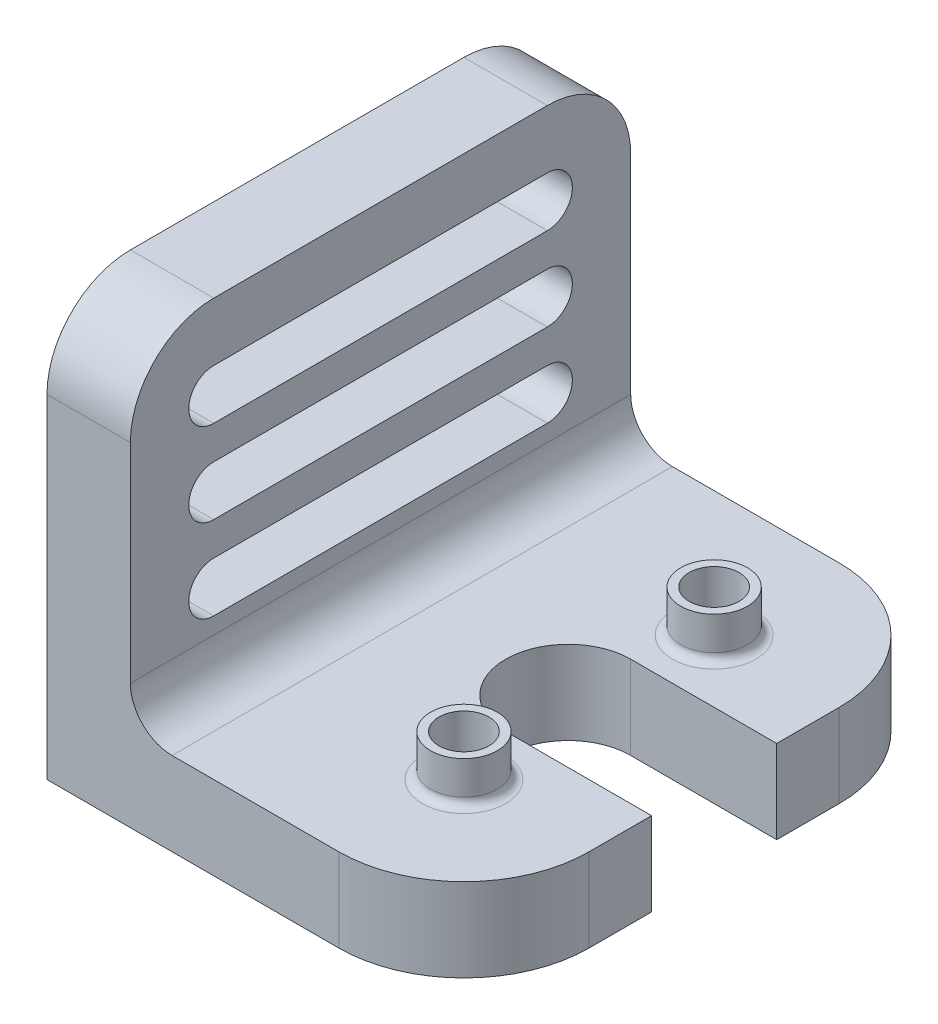
ISO-10303-21;
HEADER;
FILE_DESCRIPTION(('STEP AP214'),'2;1');
FILE_NAME('part.step','',(''),(''),'','','');
FILE_SCHEMA(('AUTOMOTIVE_DESIGN { 1 0 10303 214 1 1 1 1 }'));
ENDSEC;
DATA;
#1=APPLICATION_CONTEXT('core data for automotive mechanical design processes');
#2=APPLICATION_PROTOCOL_DEFINITION('international standard','automotive_design',2000,#1);
#3=PRODUCT_CONTEXT('',#1,'mechanical');
#4=PRODUCT('Part','Part','',(#3));
#5=PRODUCT_RELATED_PRODUCT_CATEGORY('part','',(#4));
#6=PRODUCT_DEFINITION_FORMATION('','',#4);
#7=PRODUCT_DEFINITION_CONTEXT('part definition',#1,'design');
#8=PRODUCT_DEFINITION('design','',#6,#7);
#9=PRODUCT_DEFINITION_SHAPE('','',#8);
#10=(LENGTH_UNIT() NAMED_UNIT(*) SI_UNIT(.MILLI.,.METRE.));
#11=(NAMED_UNIT(*) PLANE_ANGLE_UNIT() SI_UNIT($,.RADIAN.));
#12=(NAMED_UNIT(*) SI_UNIT($,.STERADIAN.) SOLID_ANGLE_UNIT());
#13=UNCERTAINTY_MEASURE_WITH_UNIT(LENGTH_MEASURE(1.E-05),#10,'distance_accuracy_value','');
#14=(GEOMETRIC_REPRESENTATION_CONTEXT(3) GLOBAL_UNCERTAINTY_ASSIGNED_CONTEXT((#13)) GLOBAL_UNIT_ASSIGNED_CONTEXT((#10,
#11,#12)) REPRESENTATION_CONTEXT('',''));
#15=CARTESIAN_POINT('',(0.,0.,0.));
#16=DIRECTION('',(0.,0.,1.));
#17=DIRECTION('',(1.,0.,0.));
#18=AXIS2_PLACEMENT_3D('',#15,#16,#17);
#19=CARTESIAN_POINT('',(100.,0.,60.));
#20=DIRECTION('',(-1.,0.,0.));
#21=DIRECTION('',(0.,0.,1.));
#22=AXIS2_PLACEMENT_3D('',#19,#20,#21);
#23=PLANE('',#22);
#24=DIRECTION('',(0.,0.,-1.));
#25=VECTOR('',#24,1.);
#26=CARTESIAN_POINT('',(100.,-80.,60.));
#27=LINE('',#26,#25);
#28=CARTESIAN_POINT('',(100.,-80.,-15.));
#29=VERTEX_POINT('',#28);
#30=CARTESIAN_POINT('',(100.,-80.,-30.));
#31=VERTEX_POINT('',#30);
#32=EDGE_CURVE('E357',#29,#31,#27,.T.);
#33=ORIENTED_EDGE('',*,*,#32,.F.);
#34=DIRECTION('',(0.,-1.,0.));
#35=VECTOR('',#34,1.);
#36=CARTESIAN_POINT('',(100.,0.,-15.));
#37=LINE('',#36,#35);
#38=CARTESIAN_POINT('',(100.,-100.,-15.));
#39=VERTEX_POINT('',#38);
#40=EDGE_CURVE('E427',#29,#39,#37,.T.);
#41=ORIENTED_EDGE('',*,*,#40,.T.);
#42=DIRECTION('',(0.,0.,-1.));
#43=VECTOR('',#42,1.);
#44=CARTESIAN_POINT('',(100.,-100.,60.));
#45=LINE('',#44,#43);
#46=CARTESIAN_POINT('',(100.,-100.,-30.));
#47=VERTEX_POINT('',#46);
#48=EDGE_CURVE('E375',#39,#47,#45,.T.);
#49=ORIENTED_EDGE('',*,*,#48,.T.);
#50=DIRECTION('',(0.,1.,0.));
#51=VECTOR('',#50,1.);
#52=CARTESIAN_POINT('',(100.,0.,-30.));
#53=LINE('',#52,#51);
#54=EDGE_CURVE('E394',#47,#31,#53,.T.);
#55=ORIENTED_EDGE('',*,*,#54,.T.);
#56=EDGE_LOOP('',(#33,#41,#49,#55));
#57=FACE_BOUND('',#56,.T.);
#58=ADVANCED_FACE('F41',(#57),#23,.F.);
#59=CARTESIAN_POINT('',(0.,-80.,60.));
#60=DIRECTION('',(0.,1.,0.));
#61=DIRECTION('',(0.,0.,1.));
#62=AXIS2_PLACEMENT_3D('',#59,#60,#61);
#63=PLANE('',#62);
#64=CARTESIAN_POINT('',(70.,-80.,-30.));
#65=DIRECTION('',(0.,1.,0.));
#66=DIRECTION('',(0.,0.,1.));
#67=AXIS2_PLACEMENT_3D('',#64,#65,#66);
#68=CIRCLE('',#67,10.);
#69=CARTESIAN_POINT('',(70.,-80.,-20.));
#70=VERTEX_POINT('',#69);
#71=EDGE_CURVE('E47',#70,#70,#68,.F.);
#72=ORIENTED_EDGE('',*,*,#71,.T.);
#73=EDGE_LOOP('',(#72));
#74=FACE_BOUND('',#73,.T.);
#75=CARTESIAN_POINT('',(70.,-80.,30.));
#76=DIRECTION('',(0.,1.,0.));
#77=DIRECTION('',(0.,0.,1.));
#78=AXIS2_PLACEMENT_3D('',#75,#76,#77);
#79=CIRCLE('',#78,10.);
#80=CARTESIAN_POINT('',(70.,-80.,40.));
#81=VERTEX_POINT('',#80);
#82=EDGE_CURVE('E437',#81,#81,#79,.F.);
#83=ORIENTED_EDGE('',*,*,#82,.T.);
#84=EDGE_LOOP('',(#83));
#85=FACE_BOUND('',#84,.T.);
#86=DIRECTION('',(-1.,0.,0.));
#87=VECTOR('',#86,1.);
#88=CARTESIAN_POINT('',(65.,-80.,-15.));
#89=LINE('',#88,#87);
#90=CARTESIAN_POINT('',(65.,-80.,-15.));
#91=VERTEX_POINT('',#90);
#92=EDGE_CURVE('E330',#29,#91,#89,.T.);
#93=ORIENTED_EDGE('',*,*,#92,.F.);
#94=ORIENTED_EDGE('',*,*,#32,.T.);
#95=CARTESIAN_POINT('',(70.,-80.,-30.));
#96=DIRECTION('',(0.,1.,0.));
#97=DIRECTION('',(0.,0.,1.));
#98=AXIS2_PLACEMENT_3D('',#95,#96,#97);
#99=CIRCLE('',#98,30.);
#100=CARTESIAN_POINT('',(70.,-80.,-60.));
#101=VERTEX_POINT('',#100);
#102=EDGE_CURVE('E399',#31,#101,#99,.T.);
#103=ORIENTED_EDGE('',*,*,#102,.T.);
#104=DIRECTION('',(1.,0.,0.));
#105=VECTOR('',#104,1.);
#106=CARTESIAN_POINT('',(0.,-80.,-60.));
#107=LINE('',#106,#105);
#108=CARTESIAN_POINT('',(30.0000000000001,-80.,-60.));
#109=VERTEX_POINT('',#108);
#110=EDGE_CURVE('E345',#109,#101,#107,.T.);
#111=ORIENTED_EDGE('',*,*,#110,.F.);
#112=DIRECTION('',(0.,0.,-1.));
#113=VECTOR('',#112,1.);
#114=CARTESIAN_POINT('',(30.0000000000001,-80.,60.));
#115=LINE('',#114,#113);
#116=CARTESIAN_POINT('',(30.0000000000001,-80.,60.));
#117=VERTEX_POINT('',#116);
#118=EDGE_CURVE('E389',#117,#109,#115,.T.);
#119=ORIENTED_EDGE('',*,*,#118,.F.);
#120=DIRECTION('',(1.,0.,0.));
#121=VECTOR('',#120,1.);
#122=CARTESIAN_POINT('',(0.,-80.,60.));
#123=LINE('',#122,#121);
#124=CARTESIAN_POINT('',(70.,-80.,60.));
#125=VERTEX_POINT('',#124);
#126=EDGE_CURVE('E344',#117,#125,#123,.T.);
#127=ORIENTED_EDGE('',*,*,#126,.T.);
#128=CARTESIAN_POINT('',(70.,-80.,30.));
#129=DIRECTION('',(0.,1.,0.));
#130=DIRECTION('',(0.,0.,1.));
#131=AXIS2_PLACEMENT_3D('',#128,#129,#130);
#132=CIRCLE('',#131,30.);
#133=CARTESIAN_POINT('',(100.,-80.,30.));
#134=VERTEX_POINT('',#133);
#135=EDGE_CURVE('E391',#125,#134,#132,.T.);
#136=ORIENTED_EDGE('',*,*,#135,.T.);
#137=CARTESIAN_POINT('',(100.,-80.,15.));
#138=VERTEX_POINT('',#137);
#139=EDGE_CURVE('E367',#134,#138,#27,.T.);
#140=ORIENTED_EDGE('',*,*,#139,.T.);
#141=DIRECTION('',(1.,0.,0.));
#142=VECTOR('',#141,1.);
#143=CARTESIAN_POINT('',(100.,-80.,15.));
#144=LINE('',#143,#142);
#145=CARTESIAN_POINT('',(65.,-80.,15.));
#146=VERTEX_POINT('',#145);
#147=EDGE_CURVE('E329',#146,#138,#144,.T.);
#148=ORIENTED_EDGE('',*,*,#147,.F.);
#149=CARTESIAN_POINT('',(65.,-80.,0.));
#150=DIRECTION('',(0.,1.,0.));
#151=DIRECTION('',(0.,0.,-1.));
#152=AXIS2_PLACEMENT_3D('',#149,#150,#151);
#153=CIRCLE('',#152,15.);
#154=EDGE_CURVE('E256',#91,#146,#153,.T.);
#155=ORIENTED_EDGE('',*,*,#154,.F.);
#156=EDGE_LOOP('',(#93,#94,#103,#111,#119,#127,#136,#140,#148,#155));
#157=FACE_BOUND('',#156,.T.);
#158=ADVANCED_FACE('F443',(#74,#85,#157),#63,.T.);
#159=CARTESIAN_POINT('',(30.,-70.,60.));
#160=DIRECTION('',(0.,0.,-1.));
#161=DIRECTION('',(-1.,0.,0.));
#162=AXIS2_PLACEMENT_3D('',#159,#160,#161);
#163=CYLINDRICAL_SURFACE('',#162,10.);
#164=CARTESIAN_POINT('',(30.,-70.,-60.));
#165=DIRECTION('',(0.,0.,1.));
#166=DIRECTION('',(1.,0.,0.));
#167=AXIS2_PLACEMENT_3D('',#164,#165,#166);
#168=CIRCLE('',#167,10.);
#169=CARTESIAN_POINT('',(20.,-70.,-60.));
#170=VERTEX_POINT('',#169);
#171=EDGE_CURVE('E359',#109,#170,#168,.F.);
#172=ORIENTED_EDGE('',*,*,#171,.T.);
#173=DIRECTION('',(0.,0.,-1.));
#174=VECTOR('',#173,1.);
#175=CARTESIAN_POINT('',(20.,-70.,60.));
#176=LINE('',#175,#174);
#177=CARTESIAN_POINT('',(20.,-70.,60.));
#178=VERTEX_POINT('',#177);
#179=EDGE_CURVE('E383',#178,#170,#176,.T.);
#180=ORIENTED_EDGE('',*,*,#179,.F.);
#181=CARTESIAN_POINT('',(30.,-70.,60.));
#182=DIRECTION('',(0.,0.,1.));
#183=DIRECTION('',(1.,0.,0.));
#184=AXIS2_PLACEMENT_3D('',#181,#182,#183);
#185=CIRCLE('',#184,10.);
#186=EDGE_CURVE('E348',#117,#178,#185,.F.);
#187=ORIENTED_EDGE('',*,*,#186,.F.);
#188=ORIENTED_EDGE('',*,*,#118,.T.);
#189=EDGE_LOOP('',(#172,#180,#187,#188));
#190=FACE_BOUND('',#189,.T.);
#191=ADVANCED_FACE('F501',(#190),#163,.F.);
#192=CARTESIAN_POINT('',(20.,0.,60.));
#193=DIRECTION('',(1.,0.,0.));
#194=DIRECTION('',(0.,1.,0.));
#195=AXIS2_PLACEMENT_3D('',#192,#193,#194);
#196=PLANE('',#195);
#197=CARTESIAN_POINT('',(20.,-20.,40.));
#198=DIRECTION('',(1.,0.,0.));
#199=DIRECTION('',(0.,1.,0.));
#200=AXIS2_PLACEMENT_3D('',#197,#198,#199);
#201=CIRCLE('',#200,6.);
#202=CARTESIAN_POINT('',(20.,-14.,40.));
#203=VERTEX_POINT('',#202);
#204=CARTESIAN_POINT('',(20.,-26.,40.));
#205=VERTEX_POINT('',#204);
#206=EDGE_CURVE('E57',#203,#205,#201,.T.);
#207=ORIENTED_EDGE('',*,*,#206,.F.);
#208=DIRECTION('',(0.,0.,1.));
#209=VECTOR('',#208,1.);
#210=CARTESIAN_POINT('',(20.,-14.,40.));
#211=LINE('',#210,#209);
#212=CARTESIAN_POINT('',(20.,-14.,-40.));
#213=VERTEX_POINT('',#212);
#214=EDGE_CURVE('E241',#213,#203,#211,.T.);
#215=ORIENTED_EDGE('',*,*,#214,.F.);
#216=CARTESIAN_POINT('',(20.,-20.,-40.));
#217=DIRECTION('',(1.,0.,0.));
#218=DIRECTION('',(0.,1.,0.));
#219=AXIS2_PLACEMENT_3D('',#216,#217,#218);
#220=CIRCLE('',#219,6.);
#221=CARTESIAN_POINT('',(20.,-26.,-40.));
#222=VERTEX_POINT('',#221);
#223=EDGE_CURVE('E242',#222,#213,#220,.T.);
#224=ORIENTED_EDGE('',*,*,#223,.F.);
#225=DIRECTION('',(0.,0.,-1.));
#226=VECTOR('',#225,1.);
#227=CARTESIAN_POINT('',(20.,-26.,40.));
#228=LINE('',#227,#226);
#229=EDGE_CURVE('E254',#205,#222,#228,.T.);
#230=ORIENTED_EDGE('',*,*,#229,.F.);
#231=EDGE_LOOP('',(#207,#215,#224,#230));
#232=FACE_BOUND('',#231,.T.);
#233=CARTESIAN_POINT('',(20.,-40.,39.9999999999998));
#234=DIRECTION('',(1.,0.,0.));
#235=DIRECTION('',(0.,1.,0.));
#236=AXIS2_PLACEMENT_3D('',#233,#234,#235);
#237=CIRCLE('',#236,6.);
#238=CARTESIAN_POINT('',(20.,-34.,39.9999999999998));
#239=VERTEX_POINT('',#238);
#240=CARTESIAN_POINT('',(20.,-46.,39.9999999999998));
#241=VERTEX_POINT('',#240);
#242=EDGE_CURVE('E61',#239,#241,#237,.T.);
#243=ORIENTED_EDGE('',*,*,#242,.F.);
#244=DIRECTION('',(0.,0.,1.));
#245=VECTOR('',#244,1.);
#246=CARTESIAN_POINT('',(20.,-34.,39.9999999999998));
#247=LINE('',#246,#245);
#248=CARTESIAN_POINT('',(20.,-34.,-40.0000000000002));
#249=VERTEX_POINT('',#248);
#250=EDGE_CURVE('E271',#249,#239,#247,.T.);
#251=ORIENTED_EDGE('',*,*,#250,.F.);
#252=CARTESIAN_POINT('',(20.,-40.,-40.0000000000002));
#253=DIRECTION('',(1.,0.,0.));
#254=DIRECTION('',(0.,1.,0.));
#255=AXIS2_PLACEMENT_3D('',#252,#253,#254);
#256=CIRCLE('',#255,6.);
#257=CARTESIAN_POINT('',(20.,-46.,-40.0000000000002));
#258=VERTEX_POINT('',#257);
#259=EDGE_CURVE('E277',#258,#249,#256,.T.);
#260=ORIENTED_EDGE('',*,*,#259,.F.);
#261=DIRECTION('',(0.,0.,-1.));
#262=VECTOR('',#261,1.);
#263=CARTESIAN_POINT('',(20.,-46.,39.9999999999998));
#264=LINE('',#263,#262);
#265=EDGE_CURVE('E278',#241,#258,#264,.T.);
#266=ORIENTED_EDGE('',*,*,#265,.F.);
#267=EDGE_LOOP('',(#243,#251,#260,#266));
#268=FACE_BOUND('',#267,.T.);
#269=CARTESIAN_POINT('',(20.,-60.,39.9999999999996));
#270=DIRECTION('',(1.,0.,0.));
#271=DIRECTION('',(0.,1.,0.));
#272=AXIS2_PLACEMENT_3D('',#269,#270,#271);
#273=CIRCLE('',#272,6.);
#274=CARTESIAN_POINT('',(20.,-54.,39.9999999999996));
#275=VERTEX_POINT('',#274);
#276=CARTESIAN_POINT('',(20.,-66.,39.9999999999996));
#277=VERTEX_POINT('',#276);
#278=EDGE_CURVE('E275',#275,#277,#273,.T.);
#279=ORIENTED_EDGE('',*,*,#278,.F.);
#280=DIRECTION('',(0.,0.,1.));
#281=VECTOR('',#280,1.);
#282=CARTESIAN_POINT('',(20.,-54.,39.9999999999996));
#283=LINE('',#282,#281);
#284=CARTESIAN_POINT('',(20.,-54.,-40.0000000000004));
#285=VERTEX_POINT('',#284);
#286=EDGE_CURVE('E302',#285,#275,#283,.T.);
#287=ORIENTED_EDGE('',*,*,#286,.F.);
#288=CARTESIAN_POINT('',(20.,-60.,-40.0000000000004));
#289=DIRECTION('',(1.,0.,0.));
#290=DIRECTION('',(0.,1.,0.));
#291=AXIS2_PLACEMENT_3D('',#288,#289,#290);
#292=CIRCLE('',#291,6.);
#293=CARTESIAN_POINT('',(20.,-66.,-40.0000000000004));
#294=VERTEX_POINT('',#293);
#295=EDGE_CURVE('E310',#294,#285,#292,.T.);
#296=ORIENTED_EDGE('',*,*,#295,.F.);
#297=DIRECTION('',(0.,0.,-1.));
#298=VECTOR('',#297,1.);
#299=CARTESIAN_POINT('',(20.,-66.,39.9999999999996));
#300=LINE('',#299,#298);
#301=EDGE_CURVE('E311',#277,#294,#300,.T.);
#302=ORIENTED_EDGE('',*,*,#301,.F.);
#303=EDGE_LOOP('',(#279,#287,#296,#302));
#304=FACE_BOUND('',#303,.T.);
#305=DIRECTION('',(0.,-1.,0.));
#306=VECTOR('',#305,1.);
#307=CARTESIAN_POINT('',(20.,0.,-60.));
#308=LINE('',#307,#306);
#309=CARTESIAN_POINT('',(20.,-20.,-60.));
#310=VERTEX_POINT('',#309);
#311=EDGE_CURVE('E361',#310,#170,#308,.T.);
#312=ORIENTED_EDGE('',*,*,#311,.F.);
#313=CARTESIAN_POINT('',(20.,-20.,-40.));
#314=DIRECTION('',(1.,0.,0.));
#315=DIRECTION('',(0.,1.,0.));
#316=AXIS2_PLACEMENT_3D('',#313,#314,#315);
#317=CIRCLE('',#316,20.);
#318=CARTESIAN_POINT('',(20.,0.,-40.));
#319=VERTEX_POINT('',#318);
#320=EDGE_CURVE('E415',#310,#319,#317,.T.);
#321=ORIENTED_EDGE('',*,*,#320,.T.);
#322=DIRECTION('',(0.,0.,-1.));
#323=VECTOR('',#322,1.);
#324=CARTESIAN_POINT('',(20.,0.,60.));
#325=LINE('',#324,#323);
#326=CARTESIAN_POINT('',(20.,0.,40.));
#327=VERTEX_POINT('',#326);
#328=EDGE_CURVE('E385',#327,#319,#325,.T.);
#329=ORIENTED_EDGE('',*,*,#328,.F.);
#330=CARTESIAN_POINT('',(20.,-20.,40.));
#331=DIRECTION('',(1.,0.,0.));
#332=DIRECTION('',(0.,1.,0.));
#333=AXIS2_PLACEMENT_3D('',#330,#331,#332);
#334=CIRCLE('',#333,20.);
#335=CARTESIAN_POINT('',(20.,-20.,60.));
#336=VERTEX_POINT('',#335);
#337=EDGE_CURVE('E414',#327,#336,#334,.T.);
#338=ORIENTED_EDGE('',*,*,#337,.T.);
#339=DIRECTION('',(0.,-1.,0.));
#340=VECTOR('',#339,1.);
#341=CARTESIAN_POINT('',(20.,0.,60.));
#342=LINE('',#341,#340);
#343=EDGE_CURVE('E346',#336,#178,#342,.T.);
#344=ORIENTED_EDGE('',*,*,#343,.T.);
#345=ORIENTED_EDGE('',*,*,#179,.T.);
#346=EDGE_LOOP('',(#312,#321,#329,#338,#344,#345));
#347=FACE_BOUND('',#346,.T.);
#348=ADVANCED_FACE('F573',(#232,#268,#304,#347),#196,.T.);
#349=CARTESIAN_POINT('',(0.,0.,60.));
#350=DIRECTION('',(0.,1.,0.));
#351=DIRECTION('',(0.,0.,1.));
#352=AXIS2_PLACEMENT_3D('',#349,#350,#351);
#353=PLANE('',#352);
#354=ORIENTED_EDGE('',*,*,#328,.T.);
#355=DIRECTION('',(1.,0.,0.));
#356=VECTOR('',#355,1.);
#357=CARTESIAN_POINT('',(0.,0.,-40.));
#358=LINE('',#357,#356);
#359=CARTESIAN_POINT('',(0.,0.,-40.));
#360=VERTEX_POINT('',#359);
#361=EDGE_CURVE('E416',#319,#360,#358,.F.);
#362=ORIENTED_EDGE('',*,*,#361,.T.);
#363=DIRECTION('',(0.,0.,-1.));
#364=VECTOR('',#363,1.);
#365=CARTESIAN_POINT('',(0.,0.,60.));
#366=LINE('',#365,#364);
#367=CARTESIAN_POINT('',(0.,0.,40.));
#368=VERTEX_POINT('',#367);
#369=EDGE_CURVE('E378',#368,#360,#366,.T.);
#370=ORIENTED_EDGE('',*,*,#369,.F.);
#371=DIRECTION('',(1.,0.,0.));
#372=VECTOR('',#371,1.);
#373=CARTESIAN_POINT('',(0.,0.,40.));
#374=LINE('',#373,#372);
#375=EDGE_CURVE('E417',#368,#327,#374,.T.);
#376=ORIENTED_EDGE('',*,*,#375,.T.);
#377=EDGE_LOOP('',(#354,#362,#370,#376));
#378=FACE_BOUND('',#377,.T.);
#379=ADVANCED_FACE('F550',(#378),#353,.T.);
#380=CARTESIAN_POINT('',(0.,0.,60.));
#381=DIRECTION('',(1.,0.,0.));
#382=DIRECTION('',(0.,0.,-1.));
#383=AXIS2_PLACEMENT_3D('',#380,#381,#382);
#384=PLANE('',#383);
#385=DIRECTION('',(0.,0.,1.));
#386=VECTOR('',#385,1.);
#387=CARTESIAN_POINT('',(0.,-14.,40.));
#388=LINE('',#387,#386);
#389=CARTESIAN_POINT('',(0.,-14.,-40.));
#390=VERTEX_POINT('',#389);
#391=CARTESIAN_POINT('',(0.,-14.,40.));
#392=VERTEX_POINT('',#391);
#393=EDGE_CURVE('E226',#390,#392,#388,.T.);
#394=ORIENTED_EDGE('',*,*,#393,.T.);
#395=CARTESIAN_POINT('',(0.,-20.,40.));
#396=DIRECTION('',(1.,0.,0.));
#397=DIRECTION('',(0.,1.,0.));
#398=AXIS2_PLACEMENT_3D('',#395,#396,#397);
#399=CIRCLE('',#398,6.);
#400=CARTESIAN_POINT('',(0.,-26.,40.));
#401=VERTEX_POINT('',#400);
#402=EDGE_CURVE('E224',#392,#401,#399,.T.);
#403=ORIENTED_EDGE('',*,*,#402,.T.);
#404=DIRECTION('',(0.,0.,-1.));
#405=VECTOR('',#404,1.);
#406=CARTESIAN_POINT('',(0.,-26.,40.));
#407=LINE('',#406,#405);
#408=CARTESIAN_POINT('',(0.,-26.,-40.));
#409=VERTEX_POINT('',#408);
#410=EDGE_CURVE('E235',#401,#409,#407,.T.);
#411=ORIENTED_EDGE('',*,*,#410,.T.);
#412=CARTESIAN_POINT('',(0.,-20.,-40.));
#413=DIRECTION('',(1.,0.,0.));
#414=DIRECTION('',(0.,1.,0.));
#415=AXIS2_PLACEMENT_3D('',#412,#413,#414);
#416=CIRCLE('',#415,6.);
#417=EDGE_CURVE('E236',#409,#390,#416,.T.);
#418=ORIENTED_EDGE('',*,*,#417,.T.);
#419=EDGE_LOOP('',(#394,#403,#411,#418));
#420=FACE_BOUND('',#419,.T.);
#421=DIRECTION('',(0.,0.,1.));
#422=VECTOR('',#421,1.);
#423=CARTESIAN_POINT('',(0.,-34.,39.9999999999998));
#424=LINE('',#423,#422);
#425=CARTESIAN_POINT('',(0.,-34.,-40.0000000000002));
#426=VERTEX_POINT('',#425);
#427=CARTESIAN_POINT('',(0.,-34.,39.9999999999998));
#428=VERTEX_POINT('',#427);
#429=EDGE_CURVE('E261',#426,#428,#424,.T.);
#430=ORIENTED_EDGE('',*,*,#429,.T.);
#431=CARTESIAN_POINT('',(0.,-40.,39.9999999999998));
#432=DIRECTION('',(1.,0.,0.));
#433=DIRECTION('',(0.,1.,0.));
#434=AXIS2_PLACEMENT_3D('',#431,#432,#433);
#435=CIRCLE('',#434,6.);
#436=CARTESIAN_POINT('',(0.,-46.,39.9999999999998));
#437=VERTEX_POINT('',#436);
#438=EDGE_CURVE('E280',#428,#437,#435,.T.);
#439=ORIENTED_EDGE('',*,*,#438,.T.);
#440=DIRECTION('',(0.,0.,-1.));
#441=VECTOR('',#440,1.);
#442=CARTESIAN_POINT('',(0.,-46.,39.9999999999998));
#443=LINE('',#442,#441);
#444=CARTESIAN_POINT('',(0.,-46.,-40.0000000000002));
#445=VERTEX_POINT('',#444);
#446=EDGE_CURVE('E286',#437,#445,#443,.T.);
#447=ORIENTED_EDGE('',*,*,#446,.T.);
#448=CARTESIAN_POINT('',(0.,-40.,-40.0000000000002));
#449=DIRECTION('',(1.,0.,0.));
#450=DIRECTION('',(0.,1.,0.));
#451=AXIS2_PLACEMENT_3D('',#448,#449,#450);
#452=CIRCLE('',#451,6.);
#453=EDGE_CURVE('E287',#445,#426,#452,.T.);
#454=ORIENTED_EDGE('',*,*,#453,.T.);
#455=EDGE_LOOP('',(#430,#439,#447,#454));
#456=FACE_BOUND('',#455,.T.);
#457=DIRECTION('',(0.,0.,1.));
#458=VECTOR('',#457,1.);
#459=CARTESIAN_POINT('',(0.,-54.,39.9999999999996));
#460=LINE('',#459,#458);
#461=CARTESIAN_POINT('',(0.,-54.,-40.0000000000004));
#462=VERTEX_POINT('',#461);
#463=CARTESIAN_POINT('',(0.,-54.,39.9999999999996));
#464=VERTEX_POINT('',#463);
#465=EDGE_CURVE('E300',#462,#464,#460,.T.);
#466=ORIENTED_EDGE('',*,*,#465,.T.);
#467=CARTESIAN_POINT('',(0.,-60.,39.9999999999996));
#468=DIRECTION('',(1.,0.,0.));
#469=DIRECTION('',(0.,1.,0.));
#470=AXIS2_PLACEMENT_3D('',#467,#468,#469);
#471=CIRCLE('',#470,6.);
#472=CARTESIAN_POINT('',(0.,-66.,39.9999999999996));
#473=VERTEX_POINT('',#472);
#474=EDGE_CURVE('E308',#464,#473,#471,.T.);
#475=ORIENTED_EDGE('',*,*,#474,.T.);
#476=DIRECTION('',(0.,0.,-1.));
#477=VECTOR('',#476,1.);
#478=CARTESIAN_POINT('',(0.,-66.,39.9999999999996));
#479=LINE('',#478,#477);
#480=CARTESIAN_POINT('',(0.,-66.,-40.0000000000004));
#481=VERTEX_POINT('',#480);
#482=EDGE_CURVE('E318',#473,#481,#479,.T.);
#483=ORIENTED_EDGE('',*,*,#482,.T.);
#484=CARTESIAN_POINT('',(0.,-60.,-40.0000000000004));
#485=DIRECTION('',(1.,0.,0.));
#486=DIRECTION('',(0.,1.,0.));
#487=AXIS2_PLACEMENT_3D('',#484,#485,#486);
#488=CIRCLE('',#487,6.);
#489=EDGE_CURVE('E320',#481,#462,#488,.T.);
#490=ORIENTED_EDGE('',*,*,#489,.T.);
#491=EDGE_LOOP('',(#466,#475,#483,#490));
#492=FACE_BOUND('',#491,.T.);
#493=ORIENTED_EDGE('',*,*,#369,.T.);
#494=CARTESIAN_POINT('',(0.,-20.,-40.));
#495=DIRECTION('',(1.,0.,0.));
#496=DIRECTION('',(0.,0.,-1.));
#497=AXIS2_PLACEMENT_3D('',#494,#495,#496);
#498=CIRCLE('',#497,20.);
#499=CARTESIAN_POINT('',(0.,-20.,-60.));
#500=VERTEX_POINT('',#499);
#501=EDGE_CURVE('E421',#360,#500,#498,.F.);
#502=ORIENTED_EDGE('',*,*,#501,.T.);
#503=DIRECTION('',(0.,-1.,0.));
#504=VECTOR('',#503,1.);
#505=CARTESIAN_POINT('',(0.,0.,-60.));
#506=LINE('',#505,#504);
#507=CARTESIAN_POINT('',(0.,-100.,-60.));
#508=VERTEX_POINT('',#507);
#509=EDGE_CURVE('E362',#500,#508,#506,.T.);
#510=ORIENTED_EDGE('',*,*,#509,.T.);
#511=DIRECTION('',(0.,0.,-1.));
#512=VECTOR('',#511,1.);
#513=CARTESIAN_POINT('',(0.,-100.,60.));
#514=LINE('',#513,#512);
#515=CARTESIAN_POINT('',(0.,-100.,60.));
#516=VERTEX_POINT('',#515);
#517=EDGE_CURVE('E376',#516,#508,#514,.T.);
#518=ORIENTED_EDGE('',*,*,#517,.F.);
#519=DIRECTION('',(0.,-1.,0.));
#520=VECTOR('',#519,1.);
#521=CARTESIAN_POINT('',(0.,0.,60.));
#522=LINE('',#521,#520);
#523=CARTESIAN_POINT('',(0.,-20.,60.));
#524=VERTEX_POINT('',#523);
#525=EDGE_CURVE('E354',#524,#516,#522,.T.);
#526=ORIENTED_EDGE('',*,*,#525,.F.);
#527=CARTESIAN_POINT('',(0.,-20.,40.));
#528=DIRECTION('',(1.,0.,0.));
#529=DIRECTION('',(0.,0.,-1.));
#530=AXIS2_PLACEMENT_3D('',#527,#528,#529);
#531=CIRCLE('',#530,20.);
#532=EDGE_CURVE('E423',#524,#368,#531,.F.);
#533=ORIENTED_EDGE('',*,*,#532,.T.);
#534=EDGE_LOOP('',(#493,#502,#510,#518,#526,#533));
#535=FACE_BOUND('',#534,.T.);
#536=ADVANCED_FACE('F238',(#420,#456,#492,#535),#384,.F.);
#537=CARTESIAN_POINT('',(0.,-100.,60.));
#538=DIRECTION('',(0.,1.,0.));
#539=DIRECTION('',(0.,0.,1.));
#540=AXIS2_PLACEMENT_3D('',#537,#538,#539);
#541=PLANE('',#540);
#542=ORIENTED_EDGE('',*,*,#48,.F.);
#543=DIRECTION('',(-1.,0.,0.));
#544=VECTOR('',#543,1.);
#545=CARTESIAN_POINT('',(0.,-100.,-15.));
#546=LINE('',#545,#544);
#547=CARTESIAN_POINT('',(65.,-100.,-15.));
#548=VERTEX_POINT('',#547);
#549=EDGE_CURVE('E339',#39,#548,#546,.T.);
#550=ORIENTED_EDGE('',*,*,#549,.T.);
#551=CARTESIAN_POINT('',(65.,-100.,0.));
#552=DIRECTION('',(0.,1.,0.));
#553=DIRECTION('',(0.,0.,1.));
#554=AXIS2_PLACEMENT_3D('',#551,#552,#553);
#555=CIRCLE('',#554,15.);
#556=CARTESIAN_POINT('',(65.,-100.,15.));
#557=VERTEX_POINT('',#556);
#558=EDGE_CURVE('E433',#548,#557,#555,.T.);
#559=ORIENTED_EDGE('',*,*,#558,.T.);
#560=DIRECTION('',(1.,0.,0.));
#561=VECTOR('',#560,1.);
#562=CARTESIAN_POINT('',(0.,-100.,15.));
#563=LINE('',#562,#561);
#564=CARTESIAN_POINT('',(100.,-100.,15.));
#565=VERTEX_POINT('',#564);
#566=EDGE_CURVE('E333',#557,#565,#563,.T.);
#567=ORIENTED_EDGE('',*,*,#566,.T.);
#568=CARTESIAN_POINT('',(100.,-100.,30.));
#569=VERTEX_POINT('',#568);
#570=EDGE_CURVE('E373',#569,#565,#45,.T.);
#571=ORIENTED_EDGE('',*,*,#570,.F.);
#572=CARTESIAN_POINT('',(70.,-100.,30.));
#573=DIRECTION('',(0.,1.,0.));
#574=DIRECTION('',(0.,0.,1.));
#575=AXIS2_PLACEMENT_3D('',#572,#573,#574);
#576=CIRCLE('',#575,30.);
#577=CARTESIAN_POINT('',(70.,-100.,60.));
#578=VERTEX_POINT('',#577);
#579=EDGE_CURVE('E402',#569,#578,#576,.F.);
#580=ORIENTED_EDGE('',*,*,#579,.T.);
#581=DIRECTION('',(1.,0.,0.));
#582=VECTOR('',#581,1.);
#583=CARTESIAN_POINT('',(0.,-100.,60.));
#584=LINE('',#583,#582);
#585=EDGE_CURVE('E351',#516,#578,#584,.T.);
#586=ORIENTED_EDGE('',*,*,#585,.F.);
#587=ORIENTED_EDGE('',*,*,#517,.T.);
#588=DIRECTION('',(1.,0.,0.));
#589=VECTOR('',#588,1.);
#590=CARTESIAN_POINT('',(0.,-100.,-60.));
#591=LINE('',#590,#589);
#592=CARTESIAN_POINT('',(70.,-100.,-60.));
#593=VERTEX_POINT('',#592);
#594=EDGE_CURVE('E349',#508,#593,#591,.T.);
#595=ORIENTED_EDGE('',*,*,#594,.T.);
#596=CARTESIAN_POINT('',(70.,-100.,-30.));
#597=DIRECTION('',(0.,1.,0.));
#598=DIRECTION('',(0.,0.,1.));
#599=AXIS2_PLACEMENT_3D('',#596,#597,#598);
#600=CIRCLE('',#599,30.);
#601=EDGE_CURVE('E401',#593,#47,#600,.F.);
#602=ORIENTED_EDGE('',*,*,#601,.T.);
#603=EDGE_LOOP('',(#542,#550,#559,#567,#571,#580,#586,#587,#595,#602));
#604=FACE_BOUND('',#603,.T.);
#605=ADVANCED_FACE('F507',(#604),#541,.F.);
#606=ORIENTED_EDGE('',*,*,#570,.T.);
#607=DIRECTION('',(0.,1.,0.));
#608=VECTOR('',#607,1.);
#609=CARTESIAN_POINT('',(100.,0.,15.));
#610=LINE('',#609,#608);
#611=EDGE_CURVE('E430',#565,#138,#610,.T.);
#612=ORIENTED_EDGE('',*,*,#611,.T.);
#613=ORIENTED_EDGE('',*,*,#139,.F.);
#614=DIRECTION('',(0.,1.,0.));
#615=VECTOR('',#614,1.);
#616=CARTESIAN_POINT('',(100.,-100.,30.));
#617=LINE('',#616,#615);
#618=EDGE_CURVE('E388',#134,#569,#617,.F.);
#619=ORIENTED_EDGE('',*,*,#618,.T.);
#620=EDGE_LOOP('',(#606,#612,#613,#619));
#621=FACE_BOUND('',#620,.T.);
#622=ADVANCED_FACE('F492',(#621),#23,.F.);
#623=CARTESIAN_POINT('',(0.,0.,60.));
#624=DIRECTION('',(0.,0.,1.));
#625=DIRECTION('',(1.,0.,0.));
#626=AXIS2_PLACEMENT_3D('',#623,#624,#625);
#627=PLANE('',#626);
#628=ORIENTED_EDGE('',*,*,#343,.F.);
#629=DIRECTION('',(1.,0.,0.));
#630=VECTOR('',#629,1.);
#631=CARTESIAN_POINT('',(0.,-20.,60.));
#632=LINE('',#631,#630);
#633=EDGE_CURVE('E424',#336,#524,#632,.F.);
#634=ORIENTED_EDGE('',*,*,#633,.T.);
#635=ORIENTED_EDGE('',*,*,#525,.T.);
#636=ORIENTED_EDGE('',*,*,#585,.T.);
#637=DIRECTION('',(0.,1.,0.));
#638=VECTOR('',#637,1.);
#639=CARTESIAN_POINT('',(70.,-80.,60.));
#640=LINE('',#639,#638);
#641=EDGE_CURVE('E407',#578,#125,#640,.T.);
#642=ORIENTED_EDGE('',*,*,#641,.T.);
#643=ORIENTED_EDGE('',*,*,#126,.F.);
#644=ORIENTED_EDGE('',*,*,#186,.T.);
#645=EDGE_LOOP('',(#628,#634,#635,#636,#642,#643,#644));
#646=FACE_BOUND('',#645,.T.);
#647=ADVANCED_FACE('F510',(#646),#627,.T.);
#648=CARTESIAN_POINT('',(0.,0.,-60.));
#649=DIRECTION('',(0.,0.,1.));
#650=DIRECTION('',(1.,0.,0.));
#651=AXIS2_PLACEMENT_3D('',#648,#649,#650);
#652=PLANE('',#651);
#653=ORIENTED_EDGE('',*,*,#509,.F.);
#654=DIRECTION('',(1.,0.,0.));
#655=VECTOR('',#654,1.);
#656=CARTESIAN_POINT('',(20.,-20.,-60.));
#657=LINE('',#656,#655);
#658=EDGE_CURVE('E406',#500,#310,#657,.T.);
#659=ORIENTED_EDGE('',*,*,#658,.T.);
#660=ORIENTED_EDGE('',*,*,#311,.T.);
#661=ORIENTED_EDGE('',*,*,#171,.F.);
#662=ORIENTED_EDGE('',*,*,#110,.T.);
#663=DIRECTION('',(0.,1.,0.));
#664=VECTOR('',#663,1.);
#665=CARTESIAN_POINT('',(70.,0.,-60.));
#666=LINE('',#665,#664);
#667=EDGE_CURVE('E396',#101,#593,#666,.F.);
#668=ORIENTED_EDGE('',*,*,#667,.T.);
#669=ORIENTED_EDGE('',*,*,#594,.F.);
#670=EDGE_LOOP('',(#653,#659,#660,#661,#662,#668,#669));
#671=FACE_BOUND('',#670,.T.);
#672=ADVANCED_FACE('F511',(#671),#652,.F.);
#673=CARTESIAN_POINT('',(70.,0.,-30.));
#674=DIRECTION('',(0.,1.,0.));
#675=DIRECTION('',(0.,0.,1.));
#676=AXIS2_PLACEMENT_3D('',#673,#674,#675);
#677=CYLINDRICAL_SURFACE('',#676,30.);
#678=ORIENTED_EDGE('',*,*,#601,.F.);
#679=ORIENTED_EDGE('',*,*,#667,.F.);
#680=ORIENTED_EDGE('',*,*,#102,.F.);
#681=ORIENTED_EDGE('',*,*,#54,.F.);
#682=EDGE_LOOP('',(#678,#679,#680,#681));
#683=FACE_BOUND('',#682,.T.);
#684=ADVANCED_FACE('F565',(#683),#677,.T.);
#685=CARTESIAN_POINT('',(70.,0.,30.));
#686=DIRECTION('',(0.,-1.,0.));
#687=DIRECTION('',(0.,0.,-1.));
#688=AXIS2_PLACEMENT_3D('',#685,#686,#687);
#689=CYLINDRICAL_SURFACE('',#688,30.);
#690=ORIENTED_EDGE('',*,*,#579,.F.);
#691=ORIENTED_EDGE('',*,*,#618,.F.);
#692=ORIENTED_EDGE('',*,*,#135,.F.);
#693=ORIENTED_EDGE('',*,*,#641,.F.);
#694=EDGE_LOOP('',(#690,#691,#692,#693));
#695=FACE_BOUND('',#694,.T.);
#696=ADVANCED_FACE('F527',(#695),#689,.T.);
#697=CARTESIAN_POINT('',(0.,-20.,-40.));
#698=DIRECTION('',(-1.,0.,0.));
#699=DIRECTION('',(0.,0.,1.));
#700=AXIS2_PLACEMENT_3D('',#697,#698,#699);
#701=CYLINDRICAL_SURFACE('',#700,20.);
#702=ORIENTED_EDGE('',*,*,#501,.F.);
#703=ORIENTED_EDGE('',*,*,#361,.F.);
#704=ORIENTED_EDGE('',*,*,#320,.F.);
#705=ORIENTED_EDGE('',*,*,#658,.F.);
#706=EDGE_LOOP('',(#702,#703,#704,#705));
#707=FACE_BOUND('',#706,.T.);
#708=ADVANCED_FACE('F552',(#707),#701,.T.);
#709=CARTESIAN_POINT('',(0.,-20.,40.));
#710=DIRECTION('',(1.,0.,0.));
#711=DIRECTION('',(0.,0.,-1.));
#712=AXIS2_PLACEMENT_3D('',#709,#710,#711);
#713=CYLINDRICAL_SURFACE('',#712,20.);
#714=ORIENTED_EDGE('',*,*,#532,.F.);
#715=ORIENTED_EDGE('',*,*,#633,.F.);
#716=ORIENTED_EDGE('',*,*,#337,.F.);
#717=ORIENTED_EDGE('',*,*,#375,.F.);
#718=EDGE_LOOP('',(#714,#715,#716,#717));
#719=FACE_BOUND('',#718,.T.);
#720=ADVANCED_FACE('F543',(#719),#713,.T.);
#721=CARTESIAN_POINT('',(65.,-158.,0.));
#722=DIRECTION('',(0.,1.,0.));
#723=DIRECTION('',(0.,0.,1.));
#724=AXIS2_PLACEMENT_3D('',#721,#722,#723);
#725=CYLINDRICAL_SURFACE('',#724,15.);
#726=DIRECTION('',(0.,1.,0.));
#727=VECTOR('',#726,1.);
#728=CARTESIAN_POINT('',(65.,-158.,-15.));
#729=LINE('',#728,#727);
#730=EDGE_CURVE('E335',#548,#91,#729,.T.);
#731=ORIENTED_EDGE('',*,*,#730,.T.);
#732=ORIENTED_EDGE('',*,*,#154,.T.);
#733=DIRECTION('',(0.,1.,0.));
#734=VECTOR('',#733,1.);
#735=CARTESIAN_POINT('',(65.,-158.,15.));
#736=LINE('',#735,#734);
#737=EDGE_CURVE('E334',#557,#146,#736,.T.);
#738=ORIENTED_EDGE('',*,*,#737,.F.);
#739=ORIENTED_EDGE('',*,*,#558,.F.);
#740=EDGE_LOOP('',(#731,#732,#738,#739));
#741=FACE_BOUND('',#740,.T.);
#742=ADVANCED_FACE('F567',(#741),#725,.F.);
#743=CARTESIAN_POINT('',(65.,-158.,-15.));
#744=DIRECTION('',(0.,0.,-1.));
#745=DIRECTION('',(-1.,0.,0.));
#746=AXIS2_PLACEMENT_3D('',#743,#744,#745);
#747=PLANE('',#746);
#748=ORIENTED_EDGE('',*,*,#40,.F.);
#749=ORIENTED_EDGE('',*,*,#92,.T.);
#750=ORIENTED_EDGE('',*,*,#730,.F.);
#751=ORIENTED_EDGE('',*,*,#549,.F.);
#752=EDGE_LOOP('',(#748,#749,#750,#751));
#753=FACE_BOUND('',#752,.T.);
#754=ADVANCED_FACE('F566',(#753),#747,.F.);
#755=CARTESIAN_POINT('',(100.,-158.,15.));
#756=DIRECTION('',(0.,0.,1.));
#757=DIRECTION('',(1.,0.,0.));
#758=AXIS2_PLACEMENT_3D('',#755,#756,#757);
#759=PLANE('',#758);
#760=ORIENTED_EDGE('',*,*,#737,.T.);
#761=ORIENTED_EDGE('',*,*,#147,.T.);
#762=ORIENTED_EDGE('',*,*,#611,.F.);
#763=ORIENTED_EDGE('',*,*,#566,.F.);
#764=EDGE_LOOP('',(#760,#761,#762,#763));
#765=FACE_BOUND('',#764,.T.);
#766=ADVANCED_FACE('F572',(#765),#759,.F.);
#767=CARTESIAN_POINT('',(0.,-60.,39.9999999999996));
#768=DIRECTION('',(1.,0.,0.));
#769=DIRECTION('',(0.,1.,0.));
#770=AXIS2_PLACEMENT_3D('',#767,#768,#769);
#771=CYLINDRICAL_SURFACE('',#770,6.);
#772=ORIENTED_EDGE('',*,*,#278,.T.);
#773=DIRECTION('',(1.,0.,0.));
#774=VECTOR('',#773,1.);
#775=CARTESIAN_POINT('',(0.,-66.,39.9999999999996));
#776=LINE('',#775,#774);
#777=EDGE_CURVE('E295',#473,#277,#776,.T.);
#778=ORIENTED_EDGE('',*,*,#777,.F.);
#779=ORIENTED_EDGE('',*,*,#474,.F.);
#780=DIRECTION('',(1.,0.,0.));
#781=VECTOR('',#780,1.);
#782=CARTESIAN_POINT('',(0.,-54.,39.9999999999996));
#783=LINE('',#782,#781);
#784=EDGE_CURVE('E305',#464,#275,#783,.T.);
#785=ORIENTED_EDGE('',*,*,#784,.T.);
#786=EDGE_LOOP('',(#772,#778,#779,#785));
#787=FACE_BOUND('',#786,.T.);
#788=ADVANCED_FACE('F643',(#787),#771,.F.);
#789=CARTESIAN_POINT('',(0.,-54.,39.9999999999996));
#790=DIRECTION('',(0.,1.,0.));
#791=DIRECTION('',(-1.,0.,0.));
#792=AXIS2_PLACEMENT_3D('',#789,#790,#791);
#793=PLANE('',#792);
#794=ORIENTED_EDGE('',*,*,#286,.T.);
#795=ORIENTED_EDGE('',*,*,#784,.F.);
#796=ORIENTED_EDGE('',*,*,#465,.F.);
#797=DIRECTION('',(1.,0.,0.));
#798=VECTOR('',#797,1.);
#799=CARTESIAN_POINT('',(0.,-54.,-40.0000000000004));
#800=LINE('',#799,#798);
#801=EDGE_CURVE('E297',#462,#285,#800,.T.);
#802=ORIENTED_EDGE('',*,*,#801,.T.);
#803=EDGE_LOOP('',(#794,#795,#796,#802));
#804=FACE_BOUND('',#803,.T.);
#805=ADVANCED_FACE('F652',(#804),#793,.F.);
#806=CARTESIAN_POINT('',(0.,-60.,-40.0000000000004));
#807=DIRECTION('',(1.,0.,0.));
#808=DIRECTION('',(0.,1.,0.));
#809=AXIS2_PLACEMENT_3D('',#806,#807,#808);
#810=CYLINDRICAL_SURFACE('',#809,6.);
#811=ORIENTED_EDGE('',*,*,#295,.T.);
#812=ORIENTED_EDGE('',*,*,#801,.F.);
#813=ORIENTED_EDGE('',*,*,#489,.F.);
#814=DIRECTION('',(1.,0.,0.));
#815=VECTOR('',#814,1.);
#816=CARTESIAN_POINT('',(0.,-66.,-40.0000000000004));
#817=LINE('',#816,#815);
#818=EDGE_CURVE('E296',#481,#294,#817,.T.);
#819=ORIENTED_EDGE('',*,*,#818,.T.);
#820=EDGE_LOOP('',(#811,#812,#813,#819));
#821=FACE_BOUND('',#820,.T.);
#822=ADVANCED_FACE('F661',(#821),#810,.F.);
#823=CARTESIAN_POINT('',(0.,-66.,39.9999999999996));
#824=DIRECTION('',(0.,-1.,0.));
#825=DIRECTION('',(1.,0.,0.));
#826=AXIS2_PLACEMENT_3D('',#823,#824,#825);
#827=PLANE('',#826);
#828=ORIENTED_EDGE('',*,*,#301,.T.);
#829=ORIENTED_EDGE('',*,*,#818,.F.);
#830=ORIENTED_EDGE('',*,*,#482,.F.);
#831=ORIENTED_EDGE('',*,*,#777,.T.);
#832=EDGE_LOOP('',(#828,#829,#830,#831));
#833=FACE_BOUND('',#832,.T.);
#834=ADVANCED_FACE('F672',(#833),#827,.F.);
#835=CARTESIAN_POINT('',(0.,-40.,39.9999999999998));
#836=DIRECTION('',(1.,0.,0.));
#837=DIRECTION('',(0.,1.,0.));
#838=AXIS2_PLACEMENT_3D('',#835,#836,#837);
#839=CYLINDRICAL_SURFACE('',#838,6.);
#840=ORIENTED_EDGE('',*,*,#242,.T.);
#841=DIRECTION('',(1.,0.,0.));
#842=VECTOR('',#841,1.);
#843=CARTESIAN_POINT('',(0.,-46.,39.9999999999998));
#844=LINE('',#843,#842);
#845=EDGE_CURVE('E262',#437,#241,#844,.T.);
#846=ORIENTED_EDGE('',*,*,#845,.F.);
#847=ORIENTED_EDGE('',*,*,#438,.F.);
#848=DIRECTION('',(1.,0.,0.));
#849=VECTOR('',#848,1.);
#850=CARTESIAN_POINT('',(0.,-34.,39.9999999999998));
#851=LINE('',#850,#849);
#852=EDGE_CURVE('E268',#428,#239,#851,.T.);
#853=ORIENTED_EDGE('',*,*,#852,.T.);
#854=EDGE_LOOP('',(#840,#846,#847,#853));
#855=FACE_BOUND('',#854,.T.);
#856=ADVANCED_FACE('F681',(#855),#839,.F.);
#857=CARTESIAN_POINT('',(0.,-34.,39.9999999999998));
#858=DIRECTION('',(0.,1.,0.));
#859=DIRECTION('',(-1.,0.,0.));
#860=AXIS2_PLACEMENT_3D('',#857,#858,#859);
#861=PLANE('',#860);
#862=ORIENTED_EDGE('',*,*,#250,.T.);
#863=ORIENTED_EDGE('',*,*,#852,.F.);
#864=ORIENTED_EDGE('',*,*,#429,.F.);
#865=DIRECTION('',(1.,0.,0.));
#866=VECTOR('',#865,1.);
#867=CARTESIAN_POINT('',(0.,-34.,-40.0000000000002));
#868=LINE('',#867,#866);
#869=EDGE_CURVE('E270',#426,#249,#868,.T.);
#870=ORIENTED_EDGE('',*,*,#869,.T.);
#871=EDGE_LOOP('',(#862,#863,#864,#870));
#872=FACE_BOUND('',#871,.T.);
#873=ADVANCED_FACE('F693',(#872),#861,.F.);
#874=CARTESIAN_POINT('',(0.,-40.,-40.0000000000002));
#875=DIRECTION('',(1.,0.,0.));
#876=DIRECTION('',(0.,1.,0.));
#877=AXIS2_PLACEMENT_3D('',#874,#875,#876);
#878=CYLINDRICAL_SURFACE('',#877,6.);
#879=ORIENTED_EDGE('',*,*,#259,.T.);
#880=ORIENTED_EDGE('',*,*,#869,.F.);
#881=ORIENTED_EDGE('',*,*,#453,.F.);
#882=DIRECTION('',(1.,0.,0.));
#883=VECTOR('',#882,1.);
#884=CARTESIAN_POINT('',(0.,-46.,-40.0000000000002));
#885=LINE('',#884,#883);
#886=EDGE_CURVE('E267',#445,#258,#885,.T.);
#887=ORIENTED_EDGE('',*,*,#886,.T.);
#888=EDGE_LOOP('',(#879,#880,#881,#887));
#889=FACE_BOUND('',#888,.T.);
#890=ADVANCED_FACE('F705',(#889),#878,.F.);
#891=CARTESIAN_POINT('',(0.,-46.,39.9999999999998));
#892=DIRECTION('',(0.,-1.,0.));
#893=DIRECTION('',(1.,0.,0.));
#894=AXIS2_PLACEMENT_3D('',#891,#892,#893);
#895=PLANE('',#894);
#896=ORIENTED_EDGE('',*,*,#265,.T.);
#897=ORIENTED_EDGE('',*,*,#886,.F.);
#898=ORIENTED_EDGE('',*,*,#446,.F.);
#899=ORIENTED_EDGE('',*,*,#845,.T.);
#900=EDGE_LOOP('',(#896,#897,#898,#899));
#901=FACE_BOUND('',#900,.T.);
#902=ADVANCED_FACE('F715',(#901),#895,.F.);
#903=CARTESIAN_POINT('',(0.,-20.,40.));
#904=DIRECTION('',(1.,0.,0.));
#905=DIRECTION('',(0.,1.,0.));
#906=AXIS2_PLACEMENT_3D('',#903,#904,#905);
#907=CYLINDRICAL_SURFACE('',#906,6.);
#908=ORIENTED_EDGE('',*,*,#206,.T.);
#909=DIRECTION('',(1.,0.,0.));
#910=VECTOR('',#909,1.);
#911=CARTESIAN_POINT('',(0.,-26.,40.));
#912=LINE('',#911,#910);
#913=EDGE_CURVE('E217',#401,#205,#912,.T.);
#914=ORIENTED_EDGE('',*,*,#913,.F.);
#915=ORIENTED_EDGE('',*,*,#402,.F.);
#916=DIRECTION('',(1.,0.,0.));
#917=VECTOR('',#916,1.);
#918=CARTESIAN_POINT('',(0.,-14.,40.));
#919=LINE('',#918,#917);
#920=EDGE_CURVE('E260',#392,#203,#919,.T.);
#921=ORIENTED_EDGE('',*,*,#920,.T.);
#922=EDGE_LOOP('',(#908,#914,#915,#921));
#923=FACE_BOUND('',#922,.T.);
#924=ADVANCED_FACE('F216',(#923),#907,.F.);
#925=CARTESIAN_POINT('',(0.,-14.,40.));
#926=DIRECTION('',(0.,1.,0.));
#927=DIRECTION('',(-1.,0.,0.));
#928=AXIS2_PLACEMENT_3D('',#925,#926,#927);
#929=PLANE('',#928);
#930=ORIENTED_EDGE('',*,*,#214,.T.);
#931=ORIENTED_EDGE('',*,*,#920,.F.);
#932=ORIENTED_EDGE('',*,*,#393,.F.);
#933=DIRECTION('',(1.,0.,0.));
#934=VECTOR('',#933,1.);
#935=CARTESIAN_POINT('',(0.,-14.,-40.));
#936=LINE('',#935,#934);
#937=EDGE_CURVE('E258',#390,#213,#936,.T.);
#938=ORIENTED_EDGE('',*,*,#937,.T.);
#939=EDGE_LOOP('',(#930,#931,#932,#938));
#940=FACE_BOUND('',#939,.T.);
#941=ADVANCED_FACE('F732',(#940),#929,.F.);
#942=CARTESIAN_POINT('',(0.,-20.,-40.));
#943=DIRECTION('',(1.,0.,0.));
#944=DIRECTION('',(0.,1.,0.));
#945=AXIS2_PLACEMENT_3D('',#942,#943,#944);
#946=CYLINDRICAL_SURFACE('',#945,6.);
#947=ORIENTED_EDGE('',*,*,#223,.T.);
#948=ORIENTED_EDGE('',*,*,#937,.F.);
#949=ORIENTED_EDGE('',*,*,#417,.F.);
#950=DIRECTION('',(1.,0.,0.));
#951=VECTOR('',#950,1.);
#952=CARTESIAN_POINT('',(0.,-26.,-40.));
#953=LINE('',#952,#951);
#954=EDGE_CURVE('E227',#409,#222,#953,.T.);
#955=ORIENTED_EDGE('',*,*,#954,.T.);
#956=EDGE_LOOP('',(#947,#948,#949,#955));
#957=FACE_BOUND('',#956,.T.);
#958=ADVANCED_FACE('F736',(#957),#946,.F.);
#959=CARTESIAN_POINT('',(0.,-26.,40.));
#960=DIRECTION('',(0.,-1.,0.));
#961=DIRECTION('',(1.,0.,0.));
#962=AXIS2_PLACEMENT_3D('',#959,#960,#961);
#963=PLANE('',#962);
#964=ORIENTED_EDGE('',*,*,#229,.T.);
#965=ORIENTED_EDGE('',*,*,#954,.F.);
#966=ORIENTED_EDGE('',*,*,#410,.F.);
#967=ORIENTED_EDGE('',*,*,#913,.T.);
#968=EDGE_LOOP('',(#964,#965,#966,#967));
#969=FACE_BOUND('',#968,.T.);
#970=ADVANCED_FACE('F231',(#969),#963,.F.);
#971=CARTESIAN_POINT('',(70.,-70.,-30.));
#972=DIRECTION('',(0.,-1.,0.));
#973=DIRECTION('',(0.,0.,-1.));
#974=AXIS2_PLACEMENT_3D('',#971,#972,#973);
#975=CYLINDRICAL_SURFACE('',#974,8.);
#976=CARTESIAN_POINT('',(70.,-78.,-30.));
#977=DIRECTION('',(0.,1.,0.));
#978=DIRECTION('',(0.,0.,1.));
#979=AXIS2_PLACEMENT_3D('',#976,#977,#978);
#980=CIRCLE('',#979,8.);
#981=CARTESIAN_POINT('',(70.,-78.,-22.));
#982=VERTEX_POINT('',#981);
#983=EDGE_CURVE('E436',#982,#982,#980,.T.);
#984=ORIENTED_EDGE('',*,*,#983,.T.);
#985=EDGE_LOOP('',(#984));
#986=FACE_BOUND('',#985,.T.);
#987=CARTESIAN_POINT('',(70.,-70.,-30.));
#988=DIRECTION('',(0.,1.,0.));
#989=DIRECTION('',(0.,0.,1.));
#990=AXIS2_PLACEMENT_3D('',#987,#988,#989);
#991=CIRCLE('',#990,8.);
#992=CARTESIAN_POINT('',(70.,-70.,-22.));
#993=VERTEX_POINT('',#992);
#994=EDGE_CURVE('E250',#993,#993,#991,.T.);
#995=ORIENTED_EDGE('',*,*,#994,.F.);
#996=EDGE_LOOP('',(#995));
#997=FACE_BOUND('',#996,.T.);
#998=ADVANCED_FACE('F454',(#986,#997),#975,.T.);
#999=CARTESIAN_POINT('',(70.,-70.,-30.));
#1000=DIRECTION('',(0.,1.,0.));
#1001=DIRECTION('',(0.,0.,1.));
#1002=AXIS2_PLACEMENT_3D('',#999,#1000,#1001);
#1003=PLANE('',#1002);
#1004=CARTESIAN_POINT('',(70.,-70.,-30.));
#1005=DIRECTION('',(0.,1.,0.));
#1006=DIRECTION('',(0.,0.,1.));
#1007=AXIS2_PLACEMENT_3D('',#1004,#1005,#1006);
#1008=CIRCLE('',#1007,6.);
#1009=CARTESIAN_POINT('',(70.,-70.,-24.));
#1010=VERTEX_POINT('',#1009);
#1011=EDGE_CURVE('E474',#1010,#1010,#1008,.T.);
#1012=ORIENTED_EDGE('',*,*,#1011,.F.);
#1013=EDGE_LOOP('',(#1012));
#1014=FACE_BOUND('',#1013,.T.);
#1015=ORIENTED_EDGE('',*,*,#994,.T.);
#1016=EDGE_LOOP('',(#1015));
#1017=FACE_BOUND('',#1016,.T.);
#1018=ADVANCED_FACE('F458',(#1014,#1017),#1003,.T.);
#1019=CARTESIAN_POINT('',(70.,-70.,30.));
#1020=DIRECTION('',(0.,-1.,0.));
#1021=DIRECTION('',(0.,0.,-1.));
#1022=AXIS2_PLACEMENT_3D('',#1019,#1020,#1021);
#1023=CYLINDRICAL_SURFACE('',#1022,8.);
#1024=CARTESIAN_POINT('',(70.,-78.,30.));
#1025=DIRECTION('',(0.,1.,0.));
#1026=DIRECTION('',(0.,0.,1.));
#1027=AXIS2_PLACEMENT_3D('',#1024,#1025,#1026);
#1028=CIRCLE('',#1027,8.);
#1029=CARTESIAN_POINT('',(70.,-78.,38.));
#1030=VERTEX_POINT('',#1029);
#1031=EDGE_CURVE('E11',#1030,#1030,#1028,.T.);
#1032=ORIENTED_EDGE('',*,*,#1031,.T.);
#1033=EDGE_LOOP('',(#1032));
#1034=FACE_BOUND('',#1033,.T.);
#1035=CARTESIAN_POINT('',(70.,-70.,30.));
#1036=DIRECTION('',(0.,1.,0.));
#1037=DIRECTION('',(0.,0.,1.));
#1038=AXIS2_PLACEMENT_3D('',#1035,#1036,#1037);
#1039=CIRCLE('',#1038,8.);
#1040=CARTESIAN_POINT('',(70.,-70.,38.));
#1041=VERTEX_POINT('',#1040);
#1042=EDGE_CURVE('E462',#1041,#1041,#1039,.T.);
#1043=ORIENTED_EDGE('',*,*,#1042,.F.);
#1044=EDGE_LOOP('',(#1043));
#1045=FACE_BOUND('',#1044,.T.);
#1046=ADVANCED_FACE('F484',(#1034,#1045),#1023,.T.);
#1047=CARTESIAN_POINT('',(70.,-70.,30.));
#1048=DIRECTION('',(0.,1.,0.));
#1049=DIRECTION('',(0.,0.,1.));
#1050=AXIS2_PLACEMENT_3D('',#1047,#1048,#1049);
#1051=PLANE('',#1050);
#1052=CARTESIAN_POINT('',(70.,-70.,30.));
#1053=DIRECTION('',(0.,1.,0.));
#1054=DIRECTION('',(0.,0.,1.));
#1055=AXIS2_PLACEMENT_3D('',#1052,#1053,#1054);
#1056=CIRCLE('',#1055,6.);
#1057=CARTESIAN_POINT('',(70.,-70.,36.));
#1058=VERTEX_POINT('',#1057);
#1059=EDGE_CURVE('E470',#1058,#1058,#1056,.T.);
#1060=ORIENTED_EDGE('',*,*,#1059,.F.);
#1061=EDGE_LOOP('',(#1060));
#1062=FACE_BOUND('',#1061,.T.);
#1063=ORIENTED_EDGE('',*,*,#1042,.T.);
#1064=EDGE_LOOP('',(#1063));
#1065=FACE_BOUND('',#1064,.T.);
#1066=ADVANCED_FACE('F448',(#1062,#1065),#1051,.T.);
#1067=CARTESIAN_POINT('',(70.,-78.,-30.));
#1068=DIRECTION('',(0.,1.,0.));
#1069=DIRECTION('',(0.,0.,1.));
#1070=AXIS2_PLACEMENT_3D('',#1067,#1068,#1069);
#1071=TOROIDAL_SURFACE('',#1070,10.,2.);
#1072=ORIENTED_EDGE('',*,*,#71,.F.);
#1073=EDGE_LOOP('',(#1072));
#1074=FACE_BOUND('',#1073,.T.);
#1075=ORIENTED_EDGE('',*,*,#983,.F.);
#1076=EDGE_LOOP('',(#1075));
#1077=FACE_BOUND('',#1076,.T.);
#1078=ADVANCED_FACE('F450',(#1074,#1077),#1071,.F.);
#1079=CARTESIAN_POINT('',(70.,-78.,30.));
#1080=DIRECTION('',(0.,1.,0.));
#1081=DIRECTION('',(0.,0.,1.));
#1082=AXIS2_PLACEMENT_3D('',#1079,#1080,#1081);
#1083=TOROIDAL_SURFACE('',#1082,10.,2.);
#1084=ORIENTED_EDGE('',*,*,#82,.F.);
#1085=EDGE_LOOP('',(#1084));
#1086=FACE_BOUND('',#1085,.T.);
#1087=ORIENTED_EDGE('',*,*,#1031,.F.);
#1088=EDGE_LOOP('',(#1087));
#1089=FACE_BOUND('',#1088,.T.);
#1090=ADVANCED_FACE('F43',(#1086,#1089),#1083,.F.);
#1091=CARTESIAN_POINT('',(70.,-80.,30.));
#1092=DIRECTION('',(0.,1.,0.));
#1093=DIRECTION('',(0.,0.,1.));
#1094=AXIS2_PLACEMENT_3D('',#1091,#1092,#1093);
#1095=CYLINDRICAL_SURFACE('',#1094,6.);
#1096=CARTESIAN_POINT('',(70.,-80.,30.));
#1097=DIRECTION('',(0.,1.,0.));
#1098=DIRECTION('',(0.,0.,1.));
#1099=AXIS2_PLACEMENT_3D('',#1096,#1097,#1098);
#1100=CIRCLE('',#1099,6.);
#1101=CARTESIAN_POINT('',(70.,-80.,36.));
#1102=VERTEX_POINT('',#1101);
#1103=EDGE_CURVE('E465',#1102,#1102,#1100,.T.);
#1104=ORIENTED_EDGE('',*,*,#1103,.F.);
#1105=EDGE_LOOP('',(#1104));
#1106=FACE_BOUND('',#1105,.T.);
#1107=ORIENTED_EDGE('',*,*,#1059,.T.);
#1108=EDGE_LOOP('',(#1107));
#1109=FACE_BOUND('',#1108,.T.);
#1110=ADVANCED_FACE('F480',(#1106,#1109),#1095,.F.);
#1111=CARTESIAN_POINT('',(70.,-80.,30.));
#1112=DIRECTION('',(0.,1.,0.));
#1113=DIRECTION('',(0.,0.,1.));
#1114=AXIS2_PLACEMENT_3D('',#1111,#1112,#1113);
#1115=PLANE('',#1114);
#1116=ORIENTED_EDGE('',*,*,#1103,.T.);
#1117=EDGE_LOOP('',(#1116));
#1118=FACE_BOUND('',#1117,.T.);
#1119=ADVANCED_FACE('F802',(#1118),#1115,.T.);
#1120=CARTESIAN_POINT('',(70.,-80.,-30.));
#1121=DIRECTION('',(0.,1.,0.));
#1122=DIRECTION('',(0.,0.,1.));
#1123=AXIS2_PLACEMENT_3D('',#1120,#1121,#1122);
#1124=CYLINDRICAL_SURFACE('',#1123,6.);
#1125=CARTESIAN_POINT('',(70.,-80.,-30.));
#1126=DIRECTION('',(0.,1.,0.));
#1127=DIRECTION('',(0.,0.,1.));
#1128=AXIS2_PLACEMENT_3D('',#1125,#1126,#1127);
#1129=CIRCLE('',#1128,6.);
#1130=CARTESIAN_POINT('',(70.,-80.,-24.));
#1131=VERTEX_POINT('',#1130);
#1132=EDGE_CURVE('E468',#1131,#1131,#1129,.T.);
#1133=ORIENTED_EDGE('',*,*,#1132,.F.);
#1134=EDGE_LOOP('',(#1133));
#1135=FACE_BOUND('',#1134,.T.);
#1136=ORIENTED_EDGE('',*,*,#1011,.T.);
#1137=EDGE_LOOP('',(#1136));
#1138=FACE_BOUND('',#1137,.T.);
#1139=ADVANCED_FACE('F811',(#1135,#1138),#1124,.F.);
#1140=CARTESIAN_POINT('',(70.,-80.,-30.));
#1141=DIRECTION('',(0.,1.,0.));
#1142=DIRECTION('',(0.,0.,1.));
#1143=AXIS2_PLACEMENT_3D('',#1140,#1141,#1142);
#1144=PLANE('',#1143);
#1145=ORIENTED_EDGE('',*,*,#1132,.T.);
#1146=EDGE_LOOP('',(#1145));
#1147=FACE_BOUND('',#1146,.T.);
#1148=ADVANCED_FACE('F823',(#1147),#1144,.T.);
#1149=CLOSED_SHELL('',(#58,#158,#191,#348,#379,#536,#605,#622,#647,#672,#684,#696,#708,#720,
#742,#754,#766,#788,#805,#822,#834,#856,#873,#890,#902,#924,#941,#958,#970,#998,#1018,#1046,
#1066,#1078,#1090,#1110,#1119,#1139,#1148));
#1150=MANIFOLD_SOLID_BREP('B2',#1149);
#1151=ADVANCED_BREP_SHAPE_REPRESENTATION('',(#18,#1150),#14);
#1152=SHAPE_DEFINITION_REPRESENTATION(#9,#1151);
ENDSEC;
END-ISO-10303-21;
